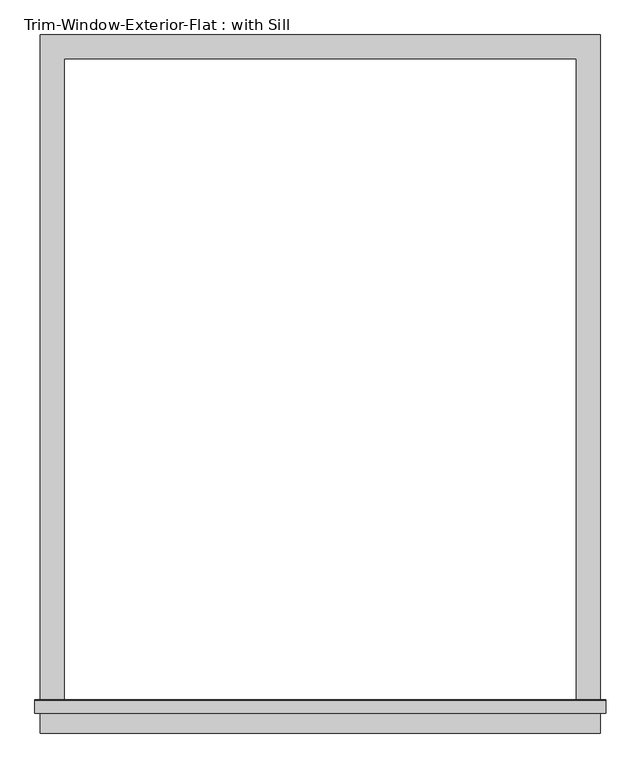
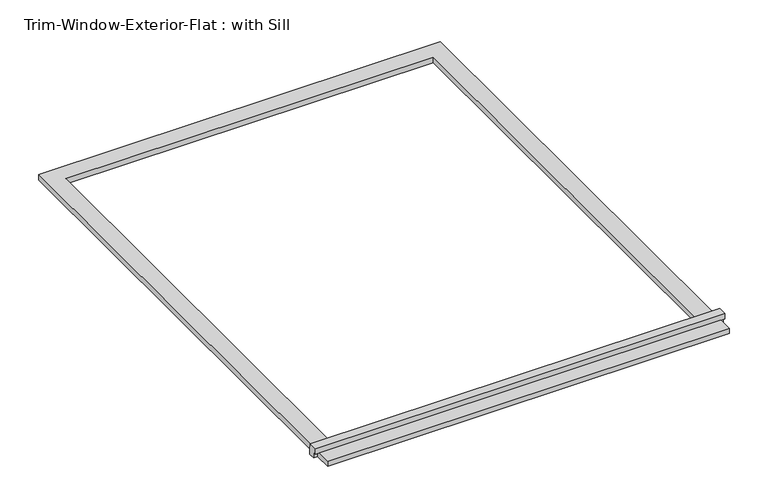
"""IFC4 building model written with IfcOpenShell, lengths in millimetres: proxy geometry, Trim-Window-Exterior-Flat : with Sill."""

from ifc_helpers import new_model, si_unit, frame, origin, origin_with_axes, place, context, project, spatial, polyline, outline, extrude, source, transform, mapped, element, save


def trim_window_exterior_flat_with_sill_92b9b949(model_context):
    return source(origin(), model_context, "Body", "SweptSolid", [
        extrude(outline(polyline([(666.75, -1546.1823709), (666.75, -1603.3323709), (-666.75, -1603.3323709), (-666.75, -1546.1823709), (666.75, -1546.1823709)])), origin_with_axes(), (0.0, 0.0, 1.0), 19.05),
        extrude(outline(polyline([(-1555.75, 38.1), (-1526.4580645, 38.1), (-1524.0, 19.05), (-1524.0, 0.0), (-1546.1823709, 0.0), (-1546.1823709, 19.05), (-1555.75, 19.05), (-1555.75, 38.1)])), frame((-679.45, 0.0, 0.0), z_axis=(1.0, 0.0, 0.0), x_axis=(0.0, 1.0, 0.0)), (0.0, 0.0, 1.0), 1358.9),
        extrude(outline(polyline([(-666.75, 57.15), (666.75, 57.15), (666.75, -1524.0), (609.6, -1524.0), (609.6, 0.0), (-609.6, 0.0), (-609.6, -1524.0), (-666.75, -1524.0), (-666.75, 57.15)])), origin_with_axes(), (0.0, 0.0, 1.0), 19.05),
    ])


if __name__ == "__main__":
    model = new_model("IFC4")
    model_context = context("Model", 3, world=origin())
    ifc_project = project(units=[si_unit("LENGTHUNIT", "METRE", prefix="MILLI")], contexts=[model_context])
    site = spatial("IfcSite", under=ifc_project)
    building = spatial("IfcBuilding", under=site)
    placement = place(None, origin())
    trim_window_exterior_flat_with_sill_shape = trim_window_exterior_flat_with_sill_92b9b949(model_context)
    element("IfcBuildingElementProxy", 1, Name="Trim-Window-Exterior-Flat : with Sill", ObjectType="Trim-Window-Exterior-Flat : with Sill", at=placement, inside=building, context=model_context, shape_type="MappedRepresentation", body=[
        mapped(trim_window_exterior_flat_with_sill_shape, transform((0.0, 0.0, 0.0), x_axis=(1.0, 0.0, 0.0), y_axis=(0.0, 1.0, 0.0), z_axis=(0.0, 0.0, 1.0))),
    ])
    save(model, "model.ifc")

# Revit data of these elements
# Type "Trim-Window-Exterior-Flat : with Sill"
#   Trim Width = 0' - 2 1/4"
#   Trim Thickness_Picture Frame = 0' - 1 1/4"
#   Trim Thickness_with Sill = 0' - 0 3/4"
#   Sill Thickness = 0' - 1 1/4"
#   Opening Width [instance default] = 2' - 0"
#   Opening Height [instance default] = 3' - 0"
#   Default Elevation = 4' - 0"
#   Sill = yes
#   Picture Frame = no
#   Trim Material [instance default] = none
# Element 1 (IfcBuildingElementProxy, "Trim-Window-Exterior-Flat : with Sill")
#   Opening Width = 4' - 0"
#   Opening Height = 5' - 0"
#   Trim Material = Clad - White
#   Materials on its faces: "Clad - White"
# Materials
#   "Clad - White": class "Wood", colour RGB 242 242 238, transparency 0, Cost = 0
